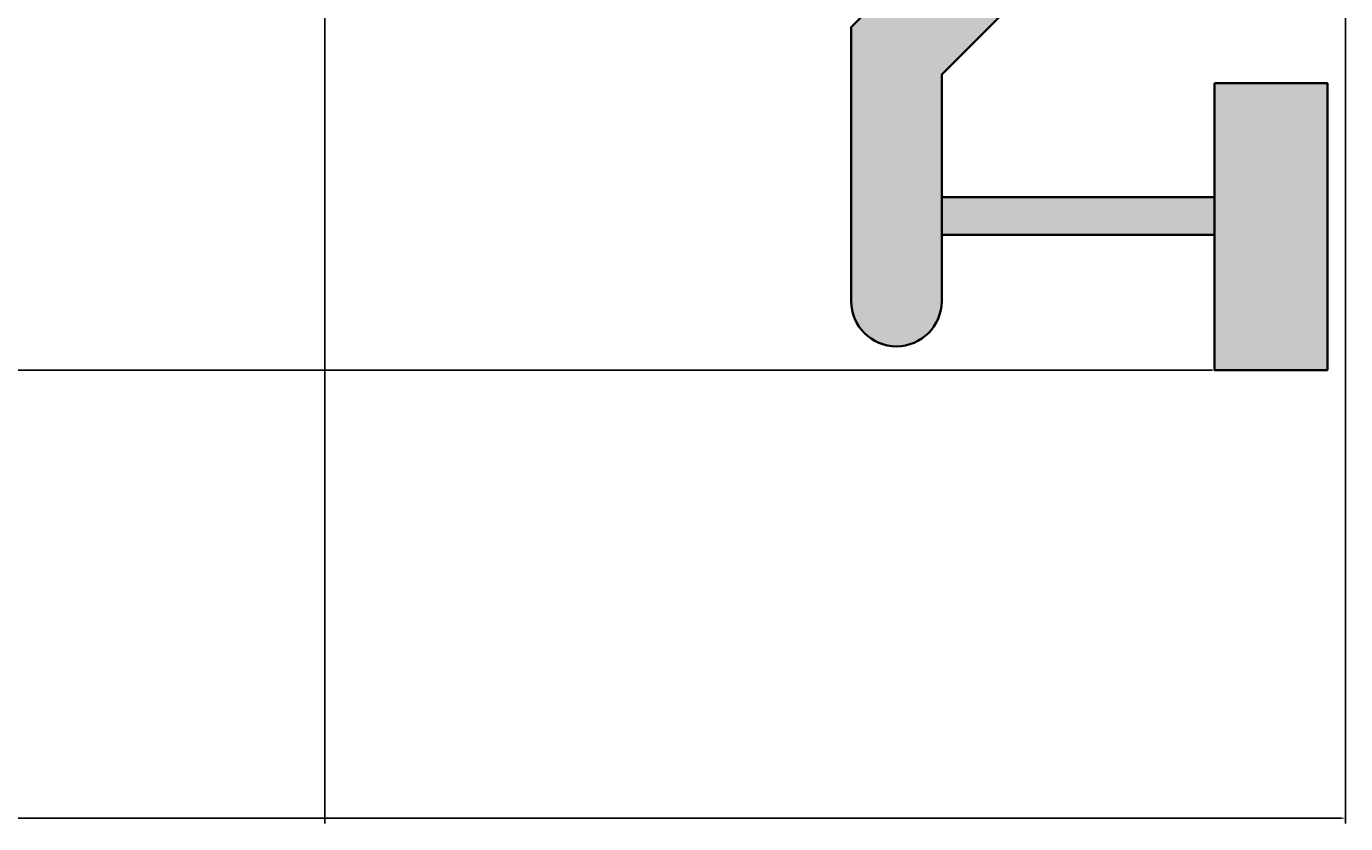
# Model space of a CAD drawing. Units: millimetres. Extents: x -11 to 280, y -4 to 208.
# Tile 35 of 55: x 222 to 266, y -4 to 23. Entities that reach past the tile are written whole.
import ezdxf

# ---------------------------------------------------------------- set-up
doc = ezdxf.new("R2010")
doc.units = ezdxf.units.MM
for name, color, linetype, lineweight in [('M-DIMS', 2, 'Continuous', 18), ('M-HYDR-CYL', 7, 'Continuous', 35), ('M-HYDR-CYL-PATT', 252, 'Continuous', 13)]:
    doc.layers.add(name, color=color, linetype=linetype, lineweight=lineweight)
doc.styles.get("Standard").update_dxf_attribs({"font": 'arial.ttf'})
doc.dimstyles.get("Standard").update_dxf_attribs({"dimtxt": 0.18, "dimasz": 0.18, "dimexe": 0.18, "dimexo": 0.0625, "dimgap": 0.09, "dimtad": 0, "dimtih": 1, "dimtoh": 1, "dimdec": 4, "dimzin": 0, "dimdsep": 46, "dimtxsty": 'Standard', "dimcen": 0.09, "dimadec": 0, "dimazin": 0, "dimtfac": 1, "dimtdec": 4, "dimtofl": 0, "dimtmove": 0, "dimatfit": 3, "dimfxl": 1, "dimtolj": 1, "dimtzin": 0, "dimarcsym": 0})

# ---------------------------------------------------------------- blocks, each defined once
blk = doc.blocks.new('*D4')
at = {"layer": 'Defpoints', "color": 0, "transparency": 16777216}
for p in [(4.763, 84.426), (266.035, 51.733), (266.035, -3.415)]:
    blk.add_point(p, dxfattribs=at)
at = {"layer": 'M-DIMS', "color": 0, "lineweight": -2, "transparency": 16777216}
for p, q in [((4.763, 84.364), (4.763, -3.595)), ((266.035, 51.67), (266.035, -3.595)), ((4.943, -3.415), (134.934, -3.415)), ((265.855, -3.415), (135.864, -3.415))]:
    blk.add_line(p, q, dxfattribs=at)
at = {"layer": 'M-DIMS', "color": 0, "transparency": 16777216}
for points in [[(4.943, -3.385), (4.943, -3.445), (4.763, -3.415)], [(265.855, -3.385), (265.855, -3.445), (266.035, -3.415)]]:
    blk.add_solid(points, dxfattribs=at)
at = {"layer": 'M-DIMS', "color": 0, "transparency": 16777216, "insert": (135.399, -3.415), "char_height": 0.18, "attachment_point": 5}
blk.add_mtext('\\A1;261.27', dxfattribs=at)
blk = doc.blocks.new('*D5')
at = {"layer": 'Defpoints', "color": 0, "transparency": 16777216}
for p in [(24.759, 192.645), (-10.087, 11.435), (261.686, 11.435)]:
    blk.add_point(p, dxfattribs=at)
at = {"layer": 'M-DIMS', "color": 0, "lineweight": -2, "transparency": 16777216}
for p, q in [((24.696, 192.645), (-10.267, 192.645)), ((-10.087, 192.465), (-10.087, 102.222)), ((-10.087, 11.615), (-10.087, 101.858)), ((261.624, 11.435), (-10.267, 11.435))]:
    blk.add_line(p, q, dxfattribs=at)
at = {"layer": 'M-DIMS', "color": 0, "transparency": 16777216}
for points in [[(-10.117, 192.465), (-10.057, 192.465), (-10.087, 192.645)], [(-10.117, 11.615), (-10.057, 11.615), (-10.087, 11.435)]]:
    blk.add_solid(points, dxfattribs=at)
at = {"layer": 'M-DIMS', "color": 0, "transparency": 16777216, "insert": (-10.087, 102.04), "char_height": 0.18, "attachment_point": 5}
blk.add_mtext('\\A1;181.2', dxfattribs=at)
blk = doc.blocks.new('*D13')
at = {"layer": 'Defpoints', "color": 0, "transparency": 16777216}
for p in [(191.774, 105.314), (232.2, 105.314), (232.2, -3.415)]:
    blk.add_point(p, dxfattribs=at)
at = {"layer": 'M-DIMS', "color": 0, "lineweight": -2, "transparency": 16777216}
for p, q in [((191.774, 105.252), (191.774, -3.595)), ((232.2, 105.252), (232.2, -3.595)), ((191.954, -3.415), (211.52, -3.415)), ((232.02, -3.415), (212.454, -3.415))]:
    blk.add_line(p, q, dxfattribs=at)
at = {"layer": 'M-DIMS', "color": 0, "transparency": 16777216}
for points in [[(191.954, -3.385), (191.954, -3.445), (191.774, -3.415)], [(232.02, -3.385), (232.02, -3.445), (232.2, -3.415)]]:
    blk.add_solid(points, dxfattribs=at)
at = {"layer": 'M-DIMS', "color": 0, "transparency": 16777216, "insert": (211.987, -3.415), "char_height": 0.18, "attachment_point": 5}
blk.add_mtext('\\A1;40.426', dxfattribs=at)

msp = doc.modelspace()

# ---------------------------------------------------------------- hatches: boundary and pattern name
at = {"layer": 'M-HYDR-CYL-PATT'}
h = msp.add_hatch(color=256, dxfattribs=at)
h.set_gradient(color1=(128, 128, 128), color2=(99, 100, 102), tint=1)
h.paths.add_polyline_path([(163.0955, 41.5991), (160.6935, 41.5991), (160.6935, 24.846), (163.0955, 24.846)])
h.paths.add_polyline_path([(259.871, 34.7226), (163.0955, 34.7226), (163.0955, 31.7226), (259.871, 31.7226, 1)])
h.paths.add_polyline_path([(257.0171, 42.0966), (265.5958, 50.6754, 1), (263.4745, 52.7967), (253.6316, 42.9537), (253.6316, 34.7226), (257.0171, 34.7226)])
h.paths.add_polyline_path([(257.0171, 25.6028), (257.0171, 31.7226), (253.6316, 31.7226), (253.6316, 26.785), (249.6456, 22.7991), (249.6456, 13.7204, 1), (252.6456, 13.7204), (252.6456, 21.2313)])
h.paths.add_polyline_path([(265.4334, 20.9382), (261.6863, 20.9382), (261.6863, 11.4346), (265.4334, 11.4346)])
h.paths.add_polyline_path([(261.6863, 17.1598), (252.6456, 17.1598), (252.6456, 15.9126), (261.6863, 15.9126)])

# ---------------------------------------------------------------- linework, layer by layer
at = {"layer": 'M-HYDR-CYL'}
for p, q in [((249.6456, 22.7991), (253.6316, 26.785)), ((257.0171, 25.6028), (252.6456, 21.2313)), ((249.6456, 13.7204), (249.6456, 22.7991)), ((252.6456, 21.2313), (252.6456, 13.7204)), ((252.6456, 17.1598), (261.6863, 17.1598)), ((252.6456, 15.9126), (261.6863, 15.9126))]:
    msp.add_line(p, q, dxfattribs=at)
msp.add_lwpolyline([(261.6863, 20.9382), (265.4334, 20.9382), (265.4334, 11.4346), (261.6863, 11.4346)], close=True, dxfattribs=at)
msp.add_arc((251.1456, 13.7204), 1.5, 180, 0, dxfattribs=at)

# ---------------------------------------------------------------- dimensions: what is measured, and where the dimension line sits
at = {"layer": 'M-DIMS'}
dim = msp.add_linear_dim(base=(-10.0865, 11.4346), p1=(24.7588, 192.645), p2=(261.6863, 11.4346), angle=90, dimstyle='Standard', override={"dimdec": 1, "dimlfac": 1, "dimrnd": 0, "dimzin": 0, "dimdsep": 46, "dimlunit": 2}, dxfattribs=at)
dim.commit()
dim.dimension.update_dxf_attribs({"geometry": '*D5', "text_midpoint": (-10.0865, 102.0398)})
for base, p1, p2, override, picture, middle in [((232.20002, -3.41542), (191.77448, 105.31407), (232.20002, 105.31407), {"dimdec": 3, "dimlfac": 1, "dimrnd": 0, "dimzin": 0, "dimdsep": 46, "dimlunit": 2}, '*D13', (211.98725, -3.41542)), ((266.0352, -3.4154), (4.7635, 84.4261), (266.0352, 51.7328), {"dimdec": 2, "dimlfac": 1, "dimrnd": 0, "dimzin": 0, "dimdsep": 46, "dimlunit": 2}, '*D4', (135.3993, -3.4154))]:
    dim = msp.add_linear_dim(base=base, p1=p1, p2=p2, dimstyle='Standard', override=override, dxfattribs=at)
    dim.commit()
    dim.dimension.update_dxf_attribs({"geometry": picture, "text_midpoint": middle})

doc.saveas('drawing.dxf')
